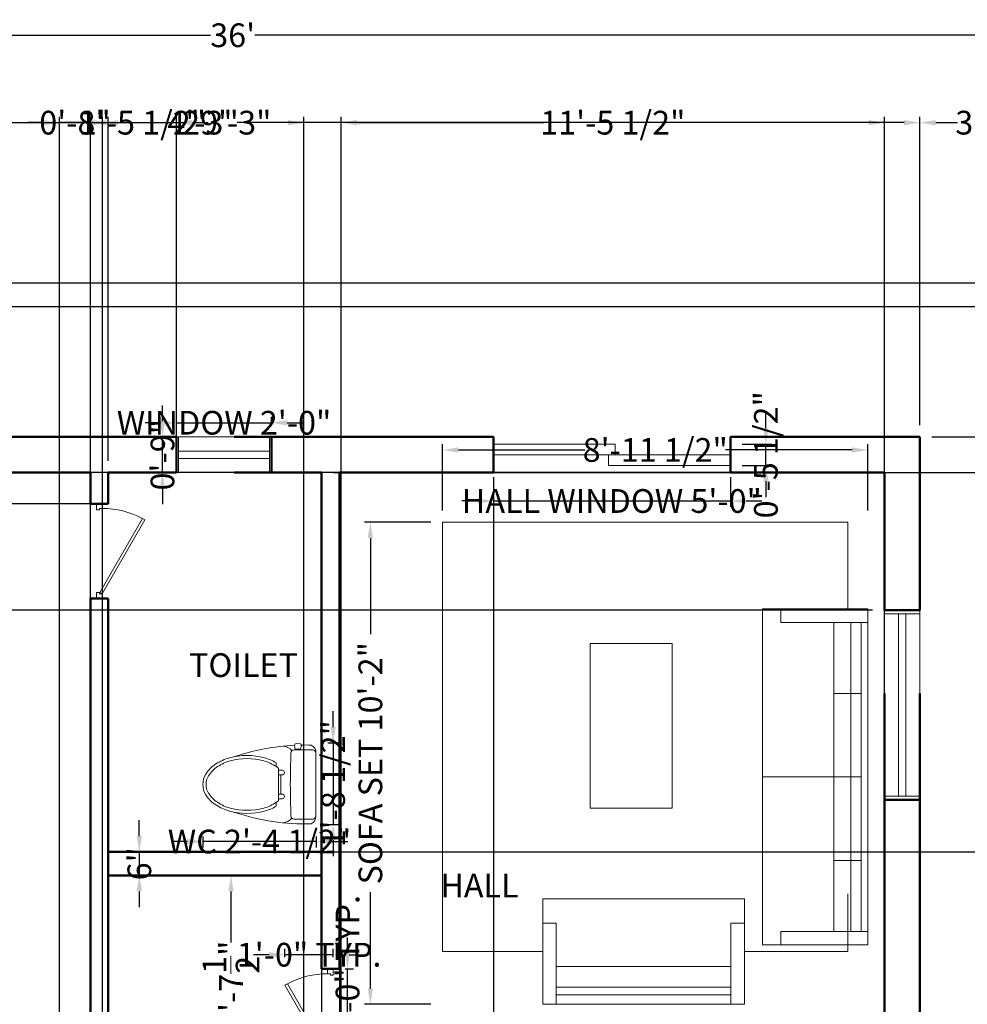
# Model space of a CAD drawing. Units: inches. Extents: x 6704 to 7574, y 11759 to 12617.
# Tile 7 of 8: x 7041 to 7281, y 12368 to 12617. Entities that reach past the tile are written whole.
import ezdxf

# ---------------------------------------------------------------- set-up
doc = ezdxf.new("R2010")
doc.units = ezdxf.units.IN
doc.header["$MEASUREMENT"] = 0
for name, color, linetype, lineweight in [('A-AREA-IDEN', 7, 'Continuous', 18), ('A-DOOR', 4, 'Continuous', 20), ('A-FLOR-FIXT', 9, 'Continuous', 18), ('A-FURN', 8, 'Continuous', 18), ('C-PROP', 7, 'Continuous', 30), ('WALL', 7, 'Continuous', 50), ('WINDOW', 2, 'Continuous', 20), ('YQ_DIM', 3, 'Continuous', 18)]:
    doc.layers.add(name, color=color, linetype=linetype, lineweight=lineweight)
doc.styles.get("Standard").update_dxf_attribs({"font": 'arial.ttf'})
doc.styles.add('YQ_DIM', font='SUPEROS.SHX', dxfattribs={"width": 0.8, "bigfont": 'HZDX.SHX'})
doc.dimstyles.new('yqi0', dxfattribs={"dimscale": 0, "dimtxt": 6, "dimasz": 4, "dimexe": 1.5, "dimexo": 3, "dimgap": 0.5, "dimtad": 0, "dimdsep": 46, "dimlunit": 4, "dimtxsty": 'Standard', "dimcen": 0, "dimclrd": 256, "dimclre": 256, "dimclrt": 7, "dimadec": 1, "dimazin": 2, "dimtfac": 1, "dimtix": 1, "dimtmove": 2, "dimatfit": 2, "dimfxl": 1, "dimtolj": 1, "dimtzin": 0, "dimarcsym": 0})

# ---------------------------------------------------------------- blocks, each defined once
blk = doc.blocks.new('*D2')
at = {"layer": 'Defpoints', "color": 0, "transparency": 16777216}
for p in [(7311.07, 12612.93), (6879.07, 12550.26), (7311.07, 12550.26)]:
    blk.add_point(p, dxfattribs=at)
at = {"layer": 'YQ_DIM', "color": 0, "lineweight": -2, "transparency": 16777216}
for p, q in [((6879.07, 12553.26), (6879.07, 12614.43)), ((7311.07, 12553.26), (7311.07, 12614.43)), ((6883.07, 12612.93), (7089.48, 12612.93)), ((7307.07, 12612.93), (7100.66, 12612.93))]:
    blk.add_line(p, q, dxfattribs=at)
at = {"layer": 'YQ_DIM', "color": 0, "transparency": 16777216}
for points in [[(6883.07, 12613.6), (6883.07, 12612.27), (6879.07, 12612.93)], [(7307.07, 12613.6), (7307.07, 12612.27), (7311.07, 12612.93)]]:
    blk.add_solid(points, dxfattribs=at)
at = {"layer": 'YQ_DIM', "color": 0, "transparency": 16777216, "insert": (7095.07, 12612.93), "char_height": 6, "attachment_point": 5}
blk.add_mtext("\\A1;36'", dxfattribs=at)
blk = doc.blocks.new('*D5')
at = {"layer": 'Defpoints', "color": 0, "transparency": 16777216}
for p in [(7090.57, 12400.26), (7090.57, 12344.76), (7094.64, 12344.76)]:
    blk.add_point(p, dxfattribs=at)
at = {"layer": 'YQ_DIM', "color": 0, "lineweight": -2, "transparency": 16777216}
for p, q in [((7093.57, 12400.26), (7096.14, 12400.26)), ((7094.64, 12396.26), (7094.64, 12383.29)), ((7094.64, 12348.76), (7094.64, 12361.72)), ((7093.57, 12344.76), (7096.14, 12344.76))]:
    blk.add_line(p, q, dxfattribs=at)
at = {"layer": 'YQ_DIM', "color": 0, "transparency": 16777216}
for points in [[(7093.97, 12396.26), (7095.31, 12396.26), (7094.64, 12400.26)], [(7093.97, 12348.76), (7095.31, 12348.76), (7094.64, 12344.76)]]:
    blk.add_solid(points, dxfattribs=at)
at = {"layer": 'YQ_DIM', "color": 0, "transparency": 16777216, "insert": (7094.64, 12372.51), "char_height": 6, "attachment_point": 5, "rotation": 90}
blk.add_mtext('\\A1;4\'-7{\\H1x;\\S1/2;}"', dxfattribs=at)
blk = doc.blocks.new('*D6')
at = {"layer": 'Defpoints', "color": 0, "transparency": 16777216}
for p in [(7071.43, 12406.26), (7071.43, 12400.26), (7071.43, 12400.26)]:
    blk.add_point(p, dxfattribs=at)
at = {"layer": 'YQ_DIM', "color": 0, "lineweight": -2, "transparency": 16777216}
for p, q in [((7071.43, 12410.26), (7071.43, 12414.26)), ((7071.43, 12406.26), (7071.43, 12400.26)), ((7074.43, 12406.26), (7072.93, 12406.26)), ((7074.43, 12400.26), (7072.93, 12400.26)), ((7071.43, 12396.26), (7071.43, 12392.26))]:
    blk.add_line(p, q, dxfattribs=at)
at = {"layer": 'YQ_DIM', "color": 0, "transparency": 16777216}
for points in [[(7070.76, 12410.26), (7072.09, 12410.26), (7071.43, 12406.26)], [(7070.76, 12396.26), (7072.09, 12396.26), (7071.43, 12400.26)]]:
    blk.add_solid(points, dxfattribs=at)
at = {"layer": 'YQ_DIM', "color": 0, "transparency": 16777216, "insert": (7071.43, 12403.26), "char_height": 6, "attachment_point": 5, "rotation": 90}
blk.add_mtext('\\A1;6"', dxfattribs=at)
blk = doc.blocks.new('WD_2TLP')
for p, q in [((-0.5, 0.3), (0.0141, 0.3)), ((0.0141, 0), (0.0141, 0.3)), ((-0.5, 0), (0.5, 0)), ((-0.0141, -0.3), (-0.0141, 0)), ((-0.0141, -0.3), (0.5, -0.3))]:
    blk.add_line(p, q)
blk = doc.blocks.new('WD_00_X1')
for p, q in [((-0.5, 0.5), (0.5, 0.5)), ((-0.48, 0.5), (-0.48, -0.5)), ((0.48, 0.5), (0.48, -0.5)), ((0.48, 0.1), (-0.48, 0.1)), ((0.48, -0.1), (-0.48, -0.1)), ((-0.5, -0.5), (0.5, -0.5))]:
    blk.add_line(p, q)
blk = doc.blocks.new('DR_CDR1')
for p, q in [((0.329, 0.48), (-0.45, 0.03)), ((-0.435, 0.004), (0.344, 0.454)), ((0.329, 0.48), (0.344, 0.454)), ((-0.45, 0.03), (-0.5, 0.03)), ((-0.435, 0.004), (-0.45, 0.03)), ((-0.45, 0.03), (-0.45, 0)), ((-0.45, 0), (-0.435, 0)), ((-0.435, 0), (-0.435, -0.03)), ((0.435, 0), (0.45, 0)), ((0.435, 0), (0.435, -0.03)), ((0.45, 0.03), (0.45, 0)), ((0.5, 0.03), (0.45, 0.03)), ((-0.435, -0.03), (-0.5, -0.03)), ((0.435, -0.03), (0.5, -0.03))]:
    blk.add_line(p, q)
blk.add_lwpolyline([(0.344, 0.454, -0.121959), (0.45, 0.03)], format="xyb")
blk = doc.blocks.new('yq_matong_01')
for p, q in [((0, 200.5), (0, -200.5)), ((20, 220.5), (138.8, 220.5)), ((252.5, 138), (252.5, 114.5)), ((215.8, 91), (238, 91)), ((238, 104.1), (238, -104.1)), ((215.8, 61), (238, 61)), ((223, 61), (223, -61)), ((215.8, -61), (238, -61)), ((215.8, -91), (238, -91)), ((252.5, -114.5), (252.5, -138)), ((20, -220.5), (138.8, -220.5)), ((97.4, -220.5), (97.4, -225.5)), ((97.4, -225.5), (131.6, -225.5)), ((131.6, -220.5), (131.6, -225.5))]:
    blk.add_line(p, q)
for centre, radius, start, end in [((54.8, 202.4), 54.8, 117.32201, 181.89921), ((63.9, -1165.4), 1416.8, 71.40679, 91.38565), ((20, 200.5), 20, 90, 180), ((138.8, 200.5), 20, 2.30634, 90), ((216.6, 161.2), 83.2, 95.49628, 139.93242), ((-4840.4, 0), 5003.3, 357.69366, 2.30634), ((406.6, -122.9), 283, 105.20877, 123.27785), ((406.6, -122.9), 303, 105.20877, 120.56985), ((439, -242.2), 426.7, 74.79123, 105.20877), ((439, -242.2), 406.7, 74.79123, 105.20877), ((471.4, -122.9), 283, 56.72215, 74.79123), ((471.4, -122.9), 303, 56.72215, 74.79123), ((520.9, -47.5), 212.8, 32.25649, 56.72215), ((215.8, 76), 15, 90, 270), ((357.1, -47.5), 192.8, 123.27785, 128.13838), ((520.9, -47.5), 192.8, 32.25649, 56.72215), ((596.2, 0), 123.8, 360, 32.25649), ((596.2, 0), 103.8, 360, 32.25649), ((215.8, -76), 15, 90, 270), ((520.9, 47.5), 192.8, 303.27785, 327.74351), ((596.2, 0), 103.8, 327.74351, 360), ((596.2, 0), 123.8, 327.74351, 360), ((357.1, 47.5), 192.8, 231.86162, 236.72215), ((406.6, 122.9), 283, 236.72215, 254.79123), ((471.4, 122.9), 283, 285.20877, 303.27785), ((520.9, 47.5), 212.8, 303.27785, 327.74351), ((63.9, 1165.4), 1416.8, 272.89667, 288.59321), ((406.6, 122.9), 303, 239.43015, 254.79123), ((439, 242.2), 426.7, 254.79123, 285.20877), ((439, 242.2), 406.7, 254.79123, 285.20877), ((471.4, 122.9), 303, 285.20877, 303.27785), ((51.3, -204.4), 51.4, 175.68696, 245.09182), ((20, -200.5), 20, 180, 270), ((156.6, -247.4), 63.1, 159.68336, 188.49388), ((72.4, -247.4), 63.1, 352.09441, 20.31664), ((138.8, -200.5), 20, 270, 357.69366), ((216.6, -161.2), 83.2, 220.06758, 264.50372), ((63.9, 1165.4), 1416.8, 268.61435, 271.20362), ((114.1, -225.6), 37, 237.52867, 304.27722)]:
    blk.add_arc(centre, radius, start, end)
blk = doc.blocks.new('SOFA 21')
for p, q in [((-49.09, -24.34), (-49.09, 0)), ((37.16, -24.34), (37.16, 0)), ((-29.27, -1.86), (-49.09, -1.86)), ((-29.27, -9.53), (-29.27, -1.86)), ((-29.27, -1.86), (-5.97, -1.86)), ((17.33, -1.86), (-5.97, -1.86)), ((-5.97, -1.86), (-5.97, -9.53)), ((17.33, -9.53), (17.33, -1.86)), ((17.33, -1.86), (37.16, -1.86)), ((37.16, -4.72), (-49.09, -4.72)), ((37.16, -9.53), (-49.09, -9.53)), ((-5.97, -9.53), (-5.97, -29.38)), ((-52.84, -24.34), (-49.09, -24.34)), ((40.91, -24.34), (37.16, -24.34)), ((-46.78, -38.24), (-46.78, -34.49)), ((-46.78, -38.24), (-69.34, -38.24)), ((-66.74, -38.24), (-66.74, -86.99)), ((-64.62, -86.99), (-64.62, -38.24)), ((-58.88, -38.24), (-58.88, -86.99)), ((-46.78, -86.99), (-69.34, -86.99)), ((-46.78, -86.99), (-46.78, -90.74))]:
    blk.add_line(p, q)
for points in [[(40.91, -29.38), (-52.84, -29.38), (-52.84, 0), (40.91, 0)], [(-69.34, -34.49), (-69.34, -90.74), (-39.97, -90.74), (-39.97, -34.49)]]:
    blk.add_lwpolyline(points, close=True)
at = {"color": 0, "linetype": 'ByBlock', "lineweight": -2}
for points in [[(-54.65, -34.49), (-54.65, -5.62)], [(-54.65, -5.62), (-38.57, -5.62)], [(40.91, -5.62), (65.11, -5.62), (65.11, -118.7), (34.12, -118.7)], [(34.12, -118.7), (-54.65, -118.7), (-54.65, -90.74)]]:
    blk.add_lwpolyline(points, dxfattribs=at)
blk.add_lwpolyline([(-14.65, -77.55), (31.25, -77.55), (31.25, -54.6), (-14.65, -54.6)], close=True, dxfattribs=at)
blk = doc.blocks.new('*D29')
at = {"layer": 'Defpoints', "color": 0, "transparency": 16777216}
for p in [(7120.54, 12376.63), (7124.14, 12376.63), (7120.54, 12352.63)]:
    blk.add_point(p, dxfattribs=at)
at = {"layer": 'YQ_DIM', "lineweight": -2, "transparency": 16777216}
for p, q in [((7124.14, 12380.63), (7124.14, 12384.63)), ((7123.54, 12376.63), (7125.64, 12376.63)), ((7124.14, 12352.63), (7124.14, 12376.63)), ((7123.54, 12352.63), (7125.64, 12352.63)), ((7124.14, 12348.63), (7124.14, 12344.63))]:
    blk.add_line(p, q, dxfattribs=at)
at = {"layer": 'YQ_DIM', "transparency": 16777216}
for points in [[(7123.48, 12380.63), (7124.81, 12380.63), (7124.14, 12376.63)], [(7123.48, 12348.63), (7124.81, 12348.63), (7124.14, 12352.63)]]:
    blk.add_solid(points, dxfattribs=at)
at = {"layer": 'YQ_DIM', "color": 7, "transparency": 16777216, "insert": (7124.14, 12364.63), "char_height": 6, "attachment_point": 5, "rotation": 90}
blk.add_mtext('\\A1;DOOR 2\'-0" TYP.', dxfattribs=at)
blk = doc.blocks.new('*D30')
at = {"layer": 'Defpoints', "color": 0, "transparency": 16777216}
for p in [(7108.3, 12380.23), (7108.3, 12376.63), (7120.54, 12376.63)]:
    blk.add_point(p, dxfattribs=at)
at = {"layer": 'YQ_DIM', "lineweight": -2, "transparency": 16777216}
for p, q in [((7104.3, 12380.23), (7100.3, 12380.23)), ((7108.3, 12379.63), (7108.3, 12381.73)), ((7120.54, 12380.23), (7108.3, 12380.23)), ((7120.54, 12379.63), (7120.54, 12381.73)), ((7124.54, 12380.23), (7128.54, 12380.23))]:
    blk.add_line(p, q, dxfattribs=at)
at = {"layer": 'YQ_DIM', "transparency": 16777216}
for points in [[(7104.3, 12380.9), (7104.3, 12379.56), (7108.3, 12380.23)], [(7124.54, 12380.9), (7124.54, 12379.56), (7120.54, 12380.23)]]:
    blk.add_solid(points, dxfattribs=at)
at = {"layer": 'YQ_DIM', "color": 7, "transparency": 16777216, "insert": (7114.42, 12380.23), "char_height": 6, "attachment_point": 5}
blk.add_mtext('\\A1;1\'-0" TYP.', dxfattribs=at)
blk = doc.blocks.new('*D33')
at = {"layer": 'Defpoints', "color": 0, "transparency": 16777216}
for p in [(7104.88, 12514.86), (7080.88, 12511.26), (7104.88, 12511.26)]:
    blk.add_point(p, dxfattribs=at)
at = {"layer": 'YQ_DIM', "lineweight": -2, "transparency": 16777216}
for p, q in [((7076.88, 12514.86), (7072.88, 12514.86)), ((7080.88, 12514.26), (7080.88, 12516.36)), ((7080.88, 12514.86), (7104.88, 12514.86)), ((7104.88, 12514.26), (7104.88, 12516.36)), ((7108.88, 12514.86), (7112.88, 12514.86))]:
    blk.add_line(p, q, dxfattribs=at)
at = {"layer": 'YQ_DIM', "transparency": 16777216}
for points in [[(7076.88, 12515.52), (7076.88, 12514.19), (7080.88, 12514.86)], [(7108.88, 12515.52), (7108.88, 12514.19), (7104.88, 12514.86)]]:
    blk.add_solid(points, dxfattribs=at)
at = {"layer": 'YQ_DIM', "color": 7, "transparency": 16777216, "insert": (7092.88, 12514.86), "char_height": 6, "attachment_point": 5}
blk.add_mtext('\\A1;WINDOW 2\'-0"', dxfattribs=at)
blk = doc.blocks.new('*D34')
at = {"layer": 'Defpoints', "color": 0, "transparency": 16777216}
for p in [(7077.28, 12511.26), (7080.88, 12511.26), (7080.88, 12502.26)]:
    blk.add_point(p, dxfattribs=at)
at = {"layer": 'YQ_DIM', "lineweight": -2, "transparency": 16777216}
for p, q in [((7077.28, 12515.26), (7077.28, 12519.26)), ((7077.88, 12511.26), (7075.78, 12511.26)), ((7077.28, 12502.26), (7077.28, 12511.26)), ((7077.88, 12502.26), (7075.78, 12502.26)), ((7077.28, 12498.26), (7077.28, 12494.26))]:
    blk.add_line(p, q, dxfattribs=at)
at = {"layer": 'YQ_DIM', "transparency": 16777216}
for points in [[(7076.61, 12515.26), (7077.95, 12515.26), (7077.28, 12511.26)], [(7076.61, 12498.26), (7077.95, 12498.26), (7077.28, 12502.26)]]:
    blk.add_solid(points, dxfattribs=at)
at = {"layer": 'YQ_DIM', "color": 7, "transparency": 16777216, "insert": (7077.28, 12506.76), "char_height": 6, "attachment_point": 5, "rotation": 90}
blk.add_mtext('\\A1;0\'-9"', dxfattribs=at)
blk = doc.blocks.new('*D35')
at = {"layer": 'Defpoints', "color": 0, "transparency": 16777216}
for p in [(7161.07, 12504.06), (7221.07, 12504.06), (7221.07, 12495.06)]:
    blk.add_point(p, dxfattribs=at)
at = {"layer": 'YQ_DIM', "lineweight": -2, "transparency": 16777216}
for p, q in [((7161.07, 12501.06), (7161.07, 12493.56)), ((7221.07, 12501.06), (7221.07, 12493.56)), ((7157.07, 12495.06), (7153.07, 12495.06)), ((7161.07, 12495.06), (7221.07, 12495.06)), ((7225.07, 12495.06), (7229.07, 12495.06))]:
    blk.add_line(p, q, dxfattribs=at)
at = {"layer": 'YQ_DIM', "transparency": 16777216}
for points in [[(7157.07, 12495.72), (7157.07, 12494.39), (7161.07, 12495.06)], [(7225.07, 12495.72), (7225.07, 12494.39), (7221.07, 12495.06)]]:
    blk.add_solid(points, dxfattribs=at)
at = {"layer": 'YQ_DIM', "color": 7, "transparency": 16777216, "insert": (7191.07, 12495.06), "char_height": 6, "attachment_point": 5}
blk.add_mtext('\\A1;HALL WINDOW 5\'-0"', dxfattribs=at)
blk = doc.blocks.new('*D36')
at = {"layer": 'Defpoints', "color": 0, "transparency": 16777216}
for p in [(7221.07, 12509.46), (7230.07, 12509.46), (7221.07, 12504.06)]:
    blk.add_point(p, dxfattribs=at)
at = {"layer": 'YQ_DIM', "lineweight": -2, "transparency": 16777216}
for p, q in [((7230.07, 12513.46), (7230.07, 12517.46)), ((7224.07, 12509.46), (7231.57, 12509.46)), ((7230.07, 12504.06), (7230.07, 12509.46)), ((7224.07, 12504.06), (7231.57, 12504.06)), ((7230.07, 12500.06), (7230.07, 12496.06))]:
    blk.add_line(p, q, dxfattribs=at)
at = {"layer": 'YQ_DIM', "transparency": 16777216}
for points in [[(7229.41, 12513.46), (7230.74, 12513.46), (7230.07, 12509.46)], [(7229.41, 12500.06), (7230.74, 12500.06), (7230.07, 12504.06)]]:
    blk.add_solid(points, dxfattribs=at)
at = {"layer": 'YQ_DIM', "color": 7, "transparency": 16777216, "insert": (7230.07, 12506.76), "char_height": 6, "attachment_point": 5, "rotation": 90}
blk.add_mtext('\\A1;0\'-5 1/2"', dxfattribs=at)
blk = doc.blocks.new('*D41')
at = {"layer": 'Defpoints', "color": 0, "transparency": 16777216}
for p in [(7129.93, 12489.68), (7148.22, 12489.68), (7148.22, 12367.72)]:
    blk.add_point(p, dxfattribs=at)
at = {"layer": 'YQ_DIM', "lineweight": -2, "transparency": 16777216}
for p, q in [((7145.22, 12489.68), (7128.43, 12489.68)), ((7129.93, 12485.68), (7129.93, 12461.39)), ((7129.93, 12371.72), (7129.93, 12396.02)), ((7145.22, 12367.72), (7128.43, 12367.72))]:
    blk.add_line(p, q, dxfattribs=at)
at = {"layer": 'YQ_DIM', "transparency": 16777216}
for points in [[(7129.26, 12485.68), (7130.6, 12485.68), (7129.93, 12489.68)], [(7129.26, 12371.72), (7130.6, 12371.72), (7129.93, 12367.72)]]:
    blk.add_solid(points, dxfattribs=at)
at = {"layer": 'YQ_DIM', "color": 7, "transparency": 16777216, "insert": (7129.93, 12428.7), "char_height": 6, "attachment_point": 5, "rotation": 90}
blk.add_mtext('\\A1;SOFA SET 10\'-2"', dxfattribs=at)
blk = doc.blocks.new('*D42')
at = {"layer": 'Defpoints', "color": 0, "transparency": 16777216}
for p in [(7255.9, 12507.98), (7148.22, 12489.68), (7255.9, 12489.68)]:
    blk.add_point(p, dxfattribs=at)
at = {"layer": 'YQ_DIM', "lineweight": -2, "transparency": 16777216}
for p, q in [((7148.22, 12492.68), (7148.22, 12509.48)), ((7255.9, 12492.68), (7255.9, 12509.48)), ((7152.22, 12507.98), (7184.26, 12507.98)), ((7251.9, 12507.98), (7219.86, 12507.98))]:
    blk.add_line(p, q, dxfattribs=at)
at = {"layer": 'YQ_DIM', "transparency": 16777216}
for points in [[(7152.22, 12508.64), (7152.22, 12507.31), (7148.22, 12507.98)], [(7251.9, 12508.64), (7251.9, 12507.31), (7255.9, 12507.98)]]:
    blk.add_solid(points, dxfattribs=at)
at = {"layer": 'YQ_DIM', "color": 7, "transparency": 16777216, "insert": (7202.06, 12507.98), "char_height": 6, "attachment_point": 5}
blk.add_mtext('\\A1;8\'-11 1/2"', dxfattribs=at)
blk = doc.blocks.new('*D43')
at = {"layer": 'Defpoints', "color": 0, "transparency": 16777216}
for p in [(7087.52, 12413.18), (7116.2, 12413.18), (7087.52, 12408.88)]:
    blk.add_point(p, dxfattribs=at)
at = {"layer": 'YQ_DIM', "lineweight": -2, "transparency": 16777216}
for p, q in [((7087.52, 12410.18), (7087.52, 12407.38)), ((7116.2, 12410.18), (7116.2, 12407.38)), ((7083.52, 12408.88), (7079.52, 12408.88)), ((7116.2, 12408.88), (7087.52, 12408.88)), ((7120.2, 12408.88), (7124.2, 12408.88))]:
    blk.add_line(p, q, dxfattribs=at)
at = {"layer": 'YQ_DIM', "transparency": 16777216}
for points in [[(7083.52, 12409.54), (7083.52, 12408.21), (7087.52, 12408.88)], [(7120.2, 12409.54), (7120.2, 12408.21), (7116.2, 12408.88)]]:
    blk.add_solid(points, dxfattribs=at)
at = {"layer": 'YQ_DIM', "color": 7, "transparency": 16777216, "insert": (7101.86, 12408.88), "char_height": 6, "attachment_point": 5}
blk.add_mtext('\\A1;WC 2\'-4 1/2"', dxfattribs=at)
blk = doc.blocks.new('*D44')
at = {"layer": 'Defpoints', "color": 0, "transparency": 16777216}
for p in [(7116.2, 12433.84), (7116.2, 12413.18), (7120.5, 12413.18)]:
    blk.add_point(p, dxfattribs=at)
at = {"layer": 'YQ_DIM', "lineweight": -2, "transparency": 16777216}
for p, q in [((7120.5, 12437.84), (7120.5, 12441.84)), ((7119.2, 12433.84), (7122, 12433.84)), ((7120.5, 12433.84), (7120.5, 12413.18)), ((7119.2, 12413.18), (7122, 12413.18)), ((7120.5, 12409.18), (7120.5, 12405.18))]:
    blk.add_line(p, q, dxfattribs=at)
at = {"layer": 'YQ_DIM', "transparency": 16777216}
for points in [[(7119.84, 12437.84), (7121.17, 12437.84), (7120.5, 12433.84)], [(7119.84, 12409.18), (7121.17, 12409.18), (7120.5, 12413.18)]]:
    blk.add_solid(points, dxfattribs=at)
at = {"layer": 'YQ_DIM', "color": 7, "transparency": 16777216, "insert": (7120.5, 12423.51), "char_height": 6, "attachment_point": 5, "rotation": 90}
blk.add_mtext('\\A1;1\'-8 1/2"', dxfattribs=at)
blk = doc.blocks.new('*D55')
at = {"layer": 'Defpoints', "color": 0, "transparency": 16777216}
for p in [(7269.07, 12590.81), (6918.07, 12511.26), (7269.07, 12511.26)]:
    blk.add_point(p, dxfattribs=at)
at = {"layer": 'YQ_DIM', "lineweight": -2, "transparency": 16777216}
for p, q in [((6918.07, 12514.26), (6918.07, 12592.31)), ((7269.07, 12514.26), (7269.07, 12592.31)), ((6922.07, 12590.81), (7082.72, 12590.81)), ((7265.07, 12590.81), (7104.43, 12590.81))]:
    blk.add_line(p, q, dxfattribs=at)
at = {"layer": 'YQ_DIM', "transparency": 16777216}
for points in [[(6922.07, 12591.47), (6922.07, 12590.14), (6918.07, 12590.81)], [(7265.07, 12591.47), (7265.07, 12590.14), (7269.07, 12590.81)]]:
    blk.add_solid(points, dxfattribs=at)
at = {"layer": 'YQ_DIM', "color": 7, "transparency": 16777216, "insert": (7093.57, 12590.81), "char_height": 6, "attachment_point": 5}
blk.add_mtext('\\A1;29\'-3"', dxfattribs=at)
blk = doc.blocks.new('*D58')
at = {"layer": 'Defpoints', "color": 0, "transparency": 16777216}
for p in [(7305.07, 12590.81), (7305.07, 12544.26), (7269.07, 12511.26)]:
    blk.add_point(p, dxfattribs=at)
at = {"layer": 'YQ_DIM', "lineweight": -2, "transparency": 16777216}
for p, q in [((7269.07, 12514.26), (7269.07, 12592.31)), ((7305.07, 12547.26), (7305.07, 12592.31)), ((7273.07, 12590.81), (7278.6, 12590.81)), ((7301.07, 12590.81), (7295.55, 12590.81))]:
    blk.add_line(p, q, dxfattribs=at)
at = {"layer": 'YQ_DIM', "transparency": 16777216}
for points in [[(7273.07, 12591.47), (7273.07, 12590.14), (7269.07, 12590.81)], [(7301.07, 12591.47), (7301.07, 12590.14), (7305.07, 12590.81)]]:
    blk.add_solid(points, dxfattribs=at)
at = {"layer": 'YQ_DIM', "color": 7, "transparency": 16777216, "insert": (7287.07, 12590.81), "char_height": 6, "attachment_point": 5}
blk.add_mtext('\\A1;3\'-0"', dxfattribs=at)
blk = doc.blocks.new('*D60')
at = {"layer": 'Defpoints', "color": 0, "transparency": 16777216}
for p in [(7063.57, 12400.26), (7117.57, 12400.26), (7117.57, 11768.08)]:
    blk.add_point(p, dxfattribs=at)
at = {"layer": 'YQ_DIM', "lineweight": -2, "transparency": 16777216}
for p, q in [((7063.57, 12397.26), (7063.57, 11766.58)), ((7117.57, 12397.26), (7117.57, 11766.58)), ((7067.57, 11768.08), (7081.98, 11768.08)), ((7113.57, 11768.08), (7099.17, 11768.08))]:
    blk.add_line(p, q, dxfattribs=at)
at = {"layer": 'YQ_DIM', "transparency": 16777216}
for points in [[(7067.57, 11768.74), (7067.57, 11767.41), (7063.57, 11768.08)], [(7113.57, 11768.74), (7113.57, 11767.41), (7117.57, 11768.08)]]:
    blk.add_solid(points, dxfattribs=at)
at = {"layer": 'YQ_DIM', "color": 7, "transparency": 16777216, "insert": (7090.57, 11768.08), "char_height": 6, "attachment_point": 5}
blk.add_mtext('\\A1;4\'-6"', dxfattribs=at)
blk = doc.blocks.new('*D61')
at = {"layer": 'Defpoints', "color": 0, "transparency": 16777216}
for p in [(7117.57, 12502.26), (7565.25, 12502.26), (7117.57, 12406.26)]:
    blk.add_point(p, dxfattribs=at)
at = {"layer": 'YQ_DIM', "lineweight": -2, "transparency": 16777216}
for p, q in [((7120.57, 12502.26), (7566.75, 12502.26)), ((7565.25, 12498.26), (7565.25, 12462.74)), ((7565.25, 12410.26), (7565.25, 12445.78)), ((7120.57, 12406.26), (7566.75, 12406.26))]:
    blk.add_line(p, q, dxfattribs=at)
at = {"layer": 'YQ_DIM', "transparency": 16777216}
for points in [[(7564.58, 12498.26), (7565.91, 12498.26), (7565.25, 12502.26)], [(7564.58, 12410.26), (7565.91, 12410.26), (7565.25, 12406.26)]]:
    blk.add_solid(points, dxfattribs=at)
at = {"layer": 'YQ_DIM', "color": 7, "transparency": 16777216, "insert": (7565.25, 12454.26), "char_height": 6, "attachment_point": 5, "rotation": 90}
blk.add_mtext('\\A1;8\'-0"', dxfattribs=at)
blk = doc.blocks.new('*D62')
at = {"layer": 'Defpoints', "color": 0, "transparency": 16777216}
for p in [(7260.07, 12419.43), (7122.07, 12340.26), (7260.07, 11768.08)]:
    blk.add_point(p, dxfattribs=at)
at = {"layer": 'YQ_DIM', "lineweight": -2, "transparency": 16777216}
for p, q in [((7260.07, 12416.43), (7260.07, 11766.58)), ((7122.07, 12337.26), (7122.07, 11766.58)), ((7126.07, 11768.08), (7180.55, 11768.08)), ((7256.07, 11768.08), (7201.6, 11768.08))]:
    blk.add_line(p, q, dxfattribs=at)
at = {"layer": 'YQ_DIM', "transparency": 16777216}
for points in [[(7126.07, 11768.74), (7126.07, 11767.41), (7122.07, 11768.08)], [(7256.07, 11768.74), (7256.07, 11767.41), (7260.07, 11768.08)]]:
    blk.add_solid(points, dxfattribs=at)
at = {"layer": 'YQ_DIM', "color": 7, "transparency": 16777216, "insert": (7191.07, 11768.08), "char_height": 6, "attachment_point": 5}
blk.add_mtext('\\A1;11\'-6"', dxfattribs=at)
blk = doc.blocks.new('*D63')
at = {"layer": 'Defpoints', "color": 0, "transparency": 16777216}
for p in [(7269.07, 12511.26), (7565.25, 12511.26), (7269.07, 12164.76)]:
    blk.add_point(p, dxfattribs=at)
at = {"layer": 'YQ_DIM', "lineweight": -2, "transparency": 16777216}
for p, q in [((7272.07, 12511.26), (7566.75, 12511.26)), ((7565.25, 12507.26), (7565.25, 12358.19)), ((7565.25, 12168.76), (7565.25, 12317.83)), ((7272.07, 12164.76), (7566.75, 12164.76))]:
    blk.add_line(p, q, dxfattribs=at)
at = {"layer": 'YQ_DIM', "transparency": 16777216}
for points in [[(7564.58, 12507.26), (7565.91, 12507.26), (7565.25, 12511.26)], [(7564.58, 12168.76), (7565.91, 12168.76), (7565.25, 12164.76)]]:
    blk.add_solid(points, dxfattribs=at)
at = {"layer": 'YQ_DIM', "color": 7, "transparency": 16777216, "insert": (7565.25, 12338.01), "char_height": 6, "attachment_point": 5, "rotation": 90}
blk.add_mtext('\\A1;28\'-10 1/2"', dxfattribs=at)
blk = doc.blocks.new('*D65')
at = {"layer": 'Defpoints', "color": 0, "transparency": 16777216}
for p in [(7113.07, 12590.81), (7062.07, 12121.26), (7113.07, 12121.26)]:
    blk.add_point(p, dxfattribs=at)
at = {"layer": 'YQ_DIM', "lineweight": -2, "transparency": 16777216}
for p, q in [((7062.07, 12124.26), (7062.07, 12592.31)), ((7113.07, 12124.26), (7113.07, 12592.31)), ((7066.07, 12590.81), (7078.98, 12590.81)), ((7109.07, 12590.81), (7096.17, 12590.81))]:
    blk.add_line(p, q, dxfattribs=at)
at = {"layer": 'YQ_DIM', "transparency": 16777216}
for points in [[(7066.07, 12591.47), (7066.07, 12590.14), (7062.07, 12590.81)], [(7109.07, 12591.47), (7109.07, 12590.14), (7113.07, 12590.81)]]:
    blk.add_solid(points, dxfattribs=at)
at = {"layer": 'YQ_DIM', "color": 7, "transparency": 16777216, "insert": (7087.57, 12590.81), "char_height": 6, "attachment_point": 5}
blk.add_mtext('\\A1;4\'-3"', dxfattribs=at)
blk = doc.blocks.new('*D76')
at = {"layer": 'Defpoints', "color": 0, "transparency": 16777216}
for p in [(7260.07, 12502.26), (6712.97, 12467.43), (7260.07, 12467.43)]:
    blk.add_point(p, dxfattribs=at)
at = {"layer": 'YQ_DIM', "lineweight": -2, "transparency": 16777216}
for p, q in [((7257.07, 12502.26), (6711.47, 12502.26)), ((6712.97, 12498.26), (6712.97, 12495.7)), ((6712.97, 12471.43), (6712.97, 12473.99)), ((7257.07, 12467.43), (6711.47, 12467.43))]:
    blk.add_line(p, q, dxfattribs=at)
at = {"layer": 'YQ_DIM', "transparency": 16777216}
for points in [[(6712.3, 12498.26), (6713.64, 12498.26), (6712.97, 12502.26)], [(6712.3, 12471.43), (6713.64, 12471.43), (6712.97, 12467.43)]]:
    blk.add_solid(points, dxfattribs=at)
at = {"layer": 'YQ_DIM', "color": 7, "transparency": 16777216, "insert": (6712.97, 12484.84), "char_height": 6, "attachment_point": 5, "rotation": 90}
blk.add_mtext('\\A1;2\'-11"', dxfattribs=at)
blk = doc.blocks.new('*D81')
at = {"layer": 'Defpoints', "color": 0, "transparency": 16777216}
for p in [(7063.57, 12502.26), (6712.97, 12494.38), (7063.57, 12494.38)]:
    blk.add_point(p, dxfattribs=at)
at = {"layer": 'YQ_DIM', "lineweight": -2, "transparency": 16777216}
for p, q in [((6712.97, 12506.26), (6712.97, 12510.26)), ((7060.57, 12502.26), (6711.47, 12502.26)), ((6712.97, 12502.26), (6712.97, 12494.38)), ((7060.57, 12494.38), (6711.47, 12494.38)), ((6712.97, 12490.38), (6712.97, 12486.38))]:
    blk.add_line(p, q, dxfattribs=at)
at = {"layer": 'YQ_DIM', "transparency": 16777216}
for points in [[(6712.3, 12506.26), (6713.64, 12506.26), (6712.97, 12502.26)], [(6712.3, 12490.38), (6713.64, 12490.38), (6712.97, 12494.38)]]:
    blk.add_solid(points, dxfattribs=at)
at = {"layer": 'YQ_DIM', "color": 7, "transparency": 16777216, "insert": (6712.97, 12498.32), "char_height": 6, "attachment_point": 5, "rotation": 90}
blk.add_mtext('\\A1;0\'-8"', dxfattribs=at)
blk = doc.blocks.new('*D83')
at = {"layer": 'Defpoints', "color": 0, "transparency": 16777216}
for p in [(7051.2, 12590.81), (7051.2, 12344.76), (7059.07, 12340.26)]:
    blk.add_point(p, dxfattribs=at)
at = {"layer": 'YQ_DIM', "lineweight": -2, "transparency": 16777216}
for p, q in [((7051.2, 12347.76), (7051.2, 12592.31)), ((7059.07, 12343.26), (7059.07, 12592.31)), ((7047.2, 12590.81), (7043.2, 12590.81)), ((7059.07, 12590.81), (7051.2, 12590.81)), ((7063.07, 12590.81), (7067.07, 12590.81))]:
    blk.add_line(p, q, dxfattribs=at)
at = {"layer": 'YQ_DIM', "transparency": 16777216}
for points in [[(7047.2, 12591.47), (7047.2, 12590.14), (7051.2, 12590.81)], [(7063.07, 12591.47), (7063.07, 12590.14), (7059.07, 12590.81)]]:
    blk.add_solid(points, dxfattribs=at)
at = {"layer": 'YQ_DIM', "color": 7, "transparency": 16777216, "insert": (7055.14, 12590.81), "char_height": 6, "attachment_point": 5}
blk.add_mtext('\\A1;0\'-8"', dxfattribs=at)
blk = doc.blocks.new('*D84')
at = {"layer": 'Defpoints', "color": 0, "transparency": 16777216}
for p in [(7080.88, 12590.81), (7063.57, 12502.26), (7080.88, 12502.26)]:
    blk.add_point(p, dxfattribs=at)
at = {"layer": 'YQ_DIM', "lineweight": -2, "transparency": 16777216}
for p, q in [((7063.57, 12505.26), (7063.57, 12592.31)), ((7080.88, 12505.26), (7080.88, 12592.31)), ((7059.57, 12590.81), (7055.57, 12590.81)), ((7063.57, 12590.81), (7080.88, 12590.81)), ((7084.88, 12590.81), (7088.88, 12590.81))]:
    blk.add_line(p, q, dxfattribs=at)
at = {"layer": 'YQ_DIM', "transparency": 16777216}
for points in [[(7059.57, 12591.47), (7059.57, 12590.14), (7063.57, 12590.81)], [(7084.88, 12591.47), (7084.88, 12590.14), (7080.88, 12590.81)]]:
    blk.add_solid(points, dxfattribs=at)
at = {"layer": 'YQ_DIM', "color": 7, "transparency": 16777216, "insert": (7072.23, 12590.81), "char_height": 6, "attachment_point": 5}
blk.add_mtext('\\A1;1\'-5 1/2"', dxfattribs=at)
blk = doc.blocks.new('*D85')
at = {"layer": 'Defpoints', "color": 0, "transparency": 16777216}
for p in [(7122.07, 12502.26), (7161.07, 12502.26), (7161.07, 11768.08)]:
    blk.add_point(p, dxfattribs=at)
at = {"layer": 'YQ_DIM', "lineweight": -2, "transparency": 16777216}
for p, q in [((7122.07, 12499.26), (7122.07, 11766.58)), ((7161.07, 12499.26), (7161.07, 11766.58)), ((7126.07, 11768.08), (7133.1, 11768.08)), ((7157.07, 11768.08), (7150.05, 11768.08))]:
    blk.add_line(p, q, dxfattribs=at)
at = {"layer": 'YQ_DIM', "transparency": 16777216}
for points in [[(7126.07, 11768.74), (7126.07, 11767.41), (7122.07, 11768.08)], [(7157.07, 11768.74), (7157.07, 11767.41), (7161.07, 11768.08)]]:
    blk.add_solid(points, dxfattribs=at)
at = {"layer": 'YQ_DIM', "color": 7, "transparency": 16777216, "insert": (7141.57, 11768.08), "char_height": 6, "attachment_point": 5}
blk.add_mtext('\\A1;3\'-3"', dxfattribs=at)
blk = doc.blocks.new('*D88')
at = {"layer": 'Defpoints', "color": 0, "transparency": 16777216}
for p in [(7260.07, 12590.81), (7260.07, 12264.3), (7122.57, 12247.15)]:
    blk.add_point(p, dxfattribs=at)
at = {"layer": 'YQ_DIM', "lineweight": -2, "transparency": 16777216}
for p, q in [((7122.57, 12250.15), (7122.57, 12592.31)), ((7260.07, 12267.3), (7260.07, 12592.31)), ((7126.57, 12590.81), (7173.81, 12590.81)), ((7256.07, 12590.81), (7208.84, 12590.81))]:
    blk.add_line(p, q, dxfattribs=at)
at = {"layer": 'YQ_DIM', "transparency": 16777216}
for points in [[(7126.57, 12591.47), (7126.57, 12590.14), (7122.57, 12590.81)], [(7256.07, 12591.47), (7256.07, 12590.14), (7260.07, 12590.81)]]:
    blk.add_solid(points, dxfattribs=at)
at = {"layer": 'YQ_DIM', "color": 7, "transparency": 16777216, "insert": (7191.32, 12590.81), "char_height": 6, "attachment_point": 5}
blk.add_mtext('\\A1;11\'-5 1/2"', dxfattribs=at)

msp = doc.modelspace()

# ---------------------------------------------------------------- linework, layer by layer
at = {"layer": 'C-PROP'}
for p, q in [((6879.073, 12550.257), (7311.073, 12550.257)), ((6885.073, 12544.257), (7305.073, 12544.257))]:
    msp.add_line(p, q, dxfattribs=at)
at = {"layer": 'WALL'}
for p, q in [((7014.823, 12511.257), (7054.573, 12511.257)), ((7054.573, 12511.257), (7080.881, 12511.257)), ((7080.881, 12502.257), (7080.881, 12511.257)), ((7095.447, 12511.257), (7117.573, 12511.257)), ((7104.881, 12502.257), (7104.881, 12511.257)), ((7108.573, 12511.257), (7161.073, 12511.257)), ((7161.073, 12511.257), (7161.073, 12502.257)), ((7221.073, 12511.257), (7269.073, 12511.257)), ((7221.073, 12511.257), (7221.073, 12502.257)), ((7269.073, 12467.428), (7269.073, 12511.257)), ((7014.823, 12502.257), (7054.573, 12502.257)), ((7054.573, 12502.257), (7059.073, 12502.257)), ((7059.073, 12494.383), (7059.073, 12502.257)), ((7063.573, 12502.257), (7080.881, 12502.257)), ((7063.573, 12494.383), (7063.573, 12502.257)), ((7095.447, 12502.257), (7117.573, 12502.257)), ((7108.573, 12502.257), (7117.573, 12502.257)), ((7117.573, 12376.631), (7117.573, 12502.257)), ((7122.073, 12502.257), (7161.073, 12502.257)), ((7122.073, 12376.631), (7122.073, 12502.257)), ((7221.073, 12502.257), (7260.073, 12502.257)), ((7260.073, 12467.428), (7260.073, 12502.257)), ((7063.573, 12494.383), (7059.073, 12494.383)), ((7059.073, 12340.257), (7059.073, 12470.383)), ((7063.573, 12470.383), (7059.073, 12470.383)), ((7063.573, 12340.257), (7063.573, 12470.383)), ((7260.073, 12467.428), (7269.073, 12467.428)), ((7260.073, 12229.631), (7260.073, 12446.383)), ((7269.073, 12229.631), (7269.073, 12446.383)), ((7260.073, 12419.428), (7269.073, 12419.428)), ((7063.573, 12406.257), (7117.573, 12406.257)), ((7063.573, 12400.257), (7117.573, 12400.257)), ((7117.573, 12376.631), (7122.073, 12376.631))]:
    msp.add_line(p, q, dxfattribs=at)

# ---------------------------------------------------------------- block references
at = {"layer": 'A-DOOR', "yscale": 24, "zscale": 24}
for p, xscale, rotation in [((7061.323, 12482.383), -24, 270), ((7119.823, 12364.631), 24, 90)]:
    msp.add_blockref('DR_CDR1', p, dxfattribs=dict(at, xscale=xscale, rotation=rotation))
at = {"layer": 'A-FLOR-FIXT', "xscale": 0.0397485514273565, "yscale": 0.0397485514273565, "zscale": 0.0397485514273565, "rotation": 180}
msp.add_blockref('yq_matong_01', (7116.136, 12423.316), dxfattribs=at)
at = {"layer": 'A-FURN', "xscale": -0.9071162186605395, "yscale": 0.9071162186605395, "zscale": 0.9071162186605395, "rotation": 270}
msp.add_blockref('SOFA 21', (7255.901, 12430.625), dxfattribs=at)
at = {"layer": 'WINDOW', "xscale": 24, "yscale": 9, "zscale": 24}
msp.add_blockref('WD_00_X1', (7092.881, 12506.757), dxfattribs=at)
at = {"layer": 'WINDOW', "yscale": 9}
for name, p, xscale, zscale, rotation in [('WD_2TLP', (7191.073, 12506.757), 60, 60, 359.9999999999983), ('WD_00_X1', (7264.573, 12443.428), 48, 48, 270)]:
    msp.add_blockref(name, p, dxfattribs=dict(at, xscale=xscale, zscale=zscale, rotation=rotation))

# ---------------------------------------------------------------- texts
at = {"layer": 'A-AREA-IDEN', "char_height": 13.77953, "attachment_point": 1, "style": 'YQ_DIM'}
for s, insert, width in [('\\pxqc;{\\H0.43543x;TOILET}', (7082.032, 12456.524), 31.54746), ('\\pxqc;{\\H0.43543x;HALL}', (7135.469, 12400.73), 44.17949)]:
    msp.add_mtext(s, dxfattribs=dict(at, insert=insert, width=width))

# ---------------------------------------------------------------- dimensions: what is measured, and where the dimension line sits
at = {"layer": 'YQ_DIM'}
for p1, p2, distance, picture, middle in [((6879.073, 12550.257), (7311.073, 12550.257), 62.676, '*D2', (7095.073, 12612.934)), ((7071.426, 12406.257), (7071.426, 12400.257), 0, '*D6', (7071.426, 12403.257)), ((7090.573, 12400.257), (7090.573, 12344.757), 4.067, '*D5', (7094.64, 12372.507))]:
    dim = msp.add_aligned_dim(p1=p1, p2=p2, distance=distance, dimstyle='yqi0', override={"dimscale": 1, "dimclrd": 0, "dimclre": 0, "dimclrt": 0}, dxfattribs=at)
    dim.commit()
    dim.dimension.update_dxf_attribs({"geometry": picture, "text_midpoint": middle})
for base, p1, p2, picture, middle in [((7080.881, 12590.807), (7063.573, 12502.257), (7080.881, 12502.257), '*D84', (7072.227, 12590.807)), ((7260.073, 12590.807), (7122.573, 12247.154), (7260.073, 12264.302), '*D88', (7191.323, 12590.807)), ((7269.073, 12590.807), (6918.073, 12511.257), (7269.073, 12511.257), '*D55', (7093.573, 12590.807)), ((7051.198, 12590.807), (7059.073, 12340.257), (7051.198, 12344.757), '*D83', (7055.135, 12590.807)), ((7113.073, 12590.807), (7062.073, 12121.257), (7113.073, 12121.257), '*D65', (7087.573, 12590.807)), ((7305.073, 12590.807), (7269.073, 12511.257), (7305.073, 12544.257), '*D58', (7287.073, 12590.807)), ((7255.901, 12507.977), (7148.224, 12489.683), (7255.901, 12489.683), '*D42', (7202.063, 12507.977)), ((7161.073, 11768.077), (7122.073, 12502.257), (7161.073, 12502.257), '*D85', (7141.573, 11768.077)), ((7260.073, 11768.077), (7122.073, 12340.257), (7260.073, 12419.428), '*D62', (7191.073, 11768.077)), ((7117.573, 11768.077), (7063.573, 12400.257), (7117.573, 12400.257), '*D60', (7090.573, 11768.077))]:
    dim = msp.add_linear_dim(base=base, p1=p1, p2=p2, dimstyle='yqi0', override={"dimscale": 1, "dimdec": 1, "dimzin": 1, "dimfrac": 2}, dxfattribs=at)
    dim.commit()
    dim.dimension.update_dxf_attribs({"geometry": picture, "text_midpoint": middle})
for base, p1, p2, text, picture, middle in [((7104.881, 12514.857), (7080.881, 12511.257), (7104.881, 12511.257), 'WINDOW <>', '*D33', (7092.881, 12514.857)), ((7221.073, 12495.057), (7161.073, 12504.057), (7221.073, 12504.057), 'HALL WINDOW <>', '*D35', (7191.073, 12495.057))]:
    dim = msp.add_linear_dim(base=base, p1=p1, p2=p2, text=text, dimstyle='yqi0', override={"dimscale": 1, "dimdec": 1, "dimzin": 1, "dimfrac": 2}, dxfattribs=at)
    dim.commit()
    dim.dimension.update_dxf_attribs({"geometry": picture, "text_midpoint": middle})
for base, p1, p2, angle, picture, middle in [((7230.073, 12509.457), (7221.073, 12504.057), (7221.073, 12509.457), 90, '*D36', (7230.073, 12506.757)), ((7077.281, 12511.257), (7080.881, 12502.257), (7080.881, 12511.257), 90, '*D34', (7077.281, 12506.757)), ((6712.97, 12494.383), (7063.573, 12502.257), (7063.573, 12494.383), 90, '*D81', (6712.97, 12498.32)), ((7565.248, 12511.257), (7269.073, 12164.757), (7269.073, 12511.257), 90, '*D63', (7565.248, 12338.007)), ((6712.97, 12467.428), (7260.073, 12502.257), (7260.073, 12467.428), 90, '*D76', (6712.97, 12484.842)), ((7565.248, 12502.257), (7117.573, 12406.257), (7117.573, 12502.257), 90, '*D61', (7565.248, 12454.257)), ((7120.503, 12413.18), (7116.2, 12433.837), (7116.2, 12413.18), 270, '*D44', (7120.503, 12423.508))]:
    dim = msp.add_linear_dim(base=base, p1=p1, p2=p2, angle=angle, dimstyle='yqi0', override={"dimscale": 1, "dimdec": 1, "dimzin": 1, "dimfrac": 2}, dxfattribs=at)
    dim.commit()
    dim.dimension.update_dxf_attribs({"geometry": picture, "text_midpoint": middle})
for base, p1, p2, angle, text, picture, middle in [((7129.93, 12489.683), (7148.224, 12367.724), (7148.224, 12489.683), 90, 'SOFA SET <>', '*D41', (7129.93, 12428.704)), ((7087.517, 12408.877), (7116.2, 12413.18), (7087.517, 12413.18), 180, 'WC <>', '*D43', (7101.859, 12408.877)), ((7124.143, 12376.631), (7120.543, 12352.631), (7120.543, 12376.631), 90, 'DOOR <> TYP.', '*D29', (7124.143, 12364.631)), ((7108.303, 12380.231), (7120.543, 12376.631), (7108.303, 12376.631), 180, '<> TYP.', '*D30', (7114.423, 12380.231))]:
    dim = msp.add_linear_dim(base=base, p1=p1, p2=p2, angle=angle, text=text, dimstyle='yqi0', override={"dimscale": 1, "dimdec": 1, "dimzin": 1, "dimfrac": 2}, dxfattribs=at)
    dim.commit()
    dim.dimension.update_dxf_attribs({"geometry": picture, "text_midpoint": middle})

doc.saveas('drawing.dxf')
